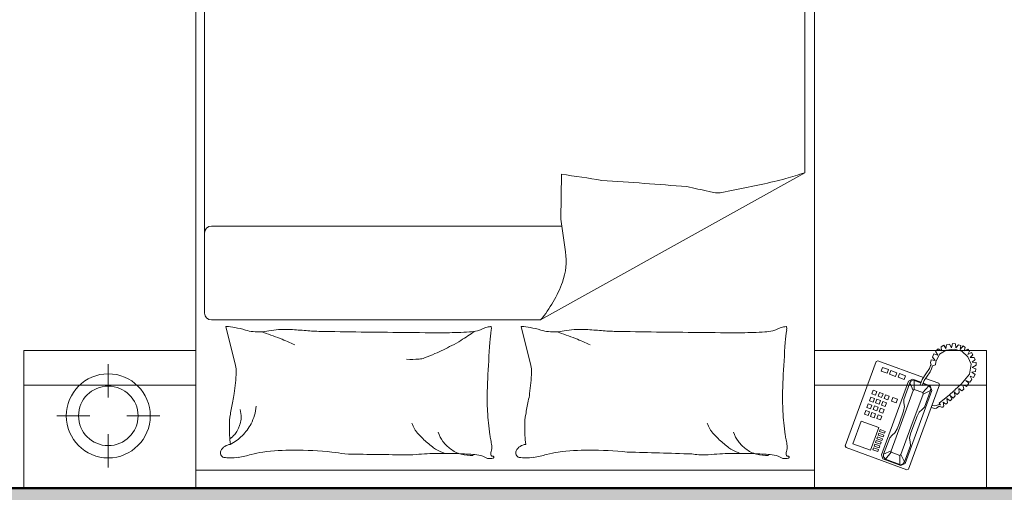
# Model space of a CAD drawing. Units: inches. Extents: x -7 to 1228, y -146 to 1091.
# Tile 45 of 88: x 81 to 169, y 574 to 616. Entities that reach past the tile are written whole.
import ezdxf

# ---------------------------------------------------------------- set-up
doc = ezdxf.new("R2010")
doc.units = ezdxf.units.IN
for name, color, linetype, lineweight in [('A-FURN', 8, 'Continuous', 18), ('A-WALL', 7, 'Continuous', 50), ('A-WALL-PATT', 251, 'Continuous', 13)]:
    doc.layers.add(name, color=color, linetype=linetype, lineweight=lineweight)
doc.styles.add('DIM_FONT', font='SIMPLEX.shx', dxfattribs={"width": 0.8})

# ---------------------------------------------------------------- blocks, each defined once
blk = doc.blocks.new('A$C4F634EDD')
for p, q in [((0, 2.6295), (0, 2.2295)), ((0.5, 2.6295), (0, 2.6295)), ((0.5, 2.6295), (2.3, 2.6295)), ((0.5, 0.5295), (0.5, 2.6295)), ((0.5, 2.2295), (0.5, 2.6295)), ((2.3, 2.6295), (2.3, 0.5295)), ((2.3, 2.6295), (2.8, 2.6295)), ((2.3, 2.2295), (2.3, 2.6295)), ((2.8, 2.6295), (2.8, 2.2295)), ((0.2457, 2.5697), (0.2457, 2.4733)), ((0.5, 2.5771), (2.3, 2.5771)), ((2.392, 2.5115), (2.5692, 2.5765)), ((2.4985, 2.5445), (2.5516, 2.564)), ((2.5062, 2.5454), (2.5487, 2.561)), ((2.5483, 2.5347), (2.5487, 2.561)), ((2.5487, 2.561), (2.5571, 2.56)), ((2.5615, 2.5536), (2.5514, 2.5318)), ((2.5516, 2.564), (2.5637, 2.5584)), ((2.5571, 2.56), (2.5615, 2.5536)), ((2.5615, 2.5536), (2.5791, 2.5058)), ((2.5637, 2.5584), (2.6418, 2.3458)), ((2.5692, 2.5765), (2.574, 2.5743)), ((2.574, 2.5743), (2.6638, 2.3298)), ((2.4842, 2.5232), (2.47, 2.518)), ((2.4862, 2.5179), (2.4842, 2.5232)), ((2.4946, 2.5331), (2.4985, 2.5445)), ((2.5734, 2.3187), (2.4946, 2.5331)), ((2.5062, 2.5454), (2.5004, 2.5392)), ((2.5004, 2.5392), (2.5013, 2.5315)), ((2.5013, 2.5315), (2.5188, 2.4836)), ((2.5013, 2.5315), (2.5231, 2.5214)), ((2.5235, 2.5256), (2.5062, 2.5454)), ((2.5231, 2.5214), (2.5235, 2.5256)), ((2.5523, 2.4417), (2.5231, 2.5214)), ((2.5483, 2.5347), (2.5235, 2.5256)), ((2.5514, 2.5318), (2.5483, 2.5347)), ((2.5807, 2.4521), (2.5514, 2.5318)), ((2.3898, 2.5066), (2.392, 2.5115)), ((2.4795, 2.2621), (2.3898, 2.5066)), ((2.412, 2.5007), (2.4634, 2.5196)), ((2.4361, 2.4352), (2.412, 2.5007)), ((2.4634, 2.5196), (2.4875, 2.454)), ((2.47, 2.518), (2.472, 2.5127)), ((2.472, 2.5127), (2.4862, 2.5179)), ((2.4881, 2.5126), (2.4739, 2.5074)), ((2.4739, 2.5074), (2.4759, 2.502)), ((2.4759, 2.502), (2.4901, 2.5073)), ((2.492, 2.5019), (2.4778, 2.4967)), ((2.4778, 2.4967), (2.4798, 2.4914)), ((2.4798, 2.4914), (2.494, 2.4966)), ((2.4901, 2.5073), (2.4881, 2.5126)), ((2.494, 2.4966), (2.492, 2.5019)), ((2.5788, 2.4956), (2.5767, 2.4848)), ((2.5791, 2.5058), (2.5788, 2.4956)), ((2.4959, 2.4913), (2.4817, 2.4861)), ((2.4817, 2.4861), (2.4837, 2.4808)), ((2.4837, 2.4808), (2.4979, 2.486)), ((2.4998, 2.4807), (2.4856, 2.4755)), ((2.4856, 2.4755), (2.4876, 2.4702)), ((2.4876, 2.4702), (2.5018, 2.4754)), ((2.5037, 2.47), (2.4895, 2.4648)), ((2.4895, 2.4648), (2.4915, 2.4595)), ((2.4915, 2.4595), (2.5057, 2.4647)), ((2.4979, 2.486), (2.4959, 2.4913)), ((2.5018, 2.4754), (2.4998, 2.4807)), ((2.5057, 2.4647), (2.5037, 2.47)), ((2.5188, 2.4836), (2.5256, 2.4761)), ((2.5256, 2.4761), (2.5342, 2.4692)), ((2.5342, 2.4692), (2.5405, 2.4574)), ((2.5767, 2.4848), (2.5795, 2.4717)), ((2.5795, 2.4717), (2.586, 2.454)), ((2.4875, 2.454), (2.4361, 2.4352)), ((2.5405, 2.4574), (2.547, 2.4397)), ((2.5594, 2.4061), (2.547, 2.4397)), ((2.5523, 2.4417), (2.5875, 2.346)), ((2.5807, 2.4521), (2.6158, 2.3564)), ((2.5984, 2.4204), (2.586, 2.454)), ((0.0957, 2.4197), (0.192, 2.4197)), ((0.2994, 2.4197), (0.3957, 2.4197)), ((2.4457, 2.4146), (2.4563, 2.4185)), ((2.4496, 2.4039), (2.4457, 2.4146)), ((2.4602, 2.4078), (2.4496, 2.4039)), ((2.4563, 2.4185), (2.4602, 2.4078)), ((2.4634, 2.4211), (2.474, 2.425)), ((2.4673, 2.4104), (2.4634, 2.4211)), ((2.4779, 2.4143), (2.4673, 2.4104)), ((2.474, 2.425), (2.4779, 2.4143)), ((2.4811, 2.4276), (2.4917, 2.4315)), ((2.485, 2.4169), (2.4811, 2.4276)), ((2.4956, 2.4208), (2.485, 2.4169)), ((2.4883, 2.4081), (2.4989, 2.412)), ((2.4922, 2.3975), (2.4883, 2.4081)), ((2.4917, 2.4315), (2.4956, 2.4208)), ((2.4989, 2.412), (2.5028, 2.4014)), ((2.5622, 2.393), (2.5594, 2.4061)), ((2.6047, 2.4086), (2.5984, 2.4204)), ((2.6133, 2.4017), (2.6047, 2.4086)), ((2.4528, 2.3951), (2.4635, 2.399)), ((2.4567, 2.3844), (2.4528, 2.3951)), ((2.4674, 2.3883), (2.4567, 2.3844)), ((2.46, 2.3756), (2.4706, 2.3795)), ((2.4635, 2.399), (2.4674, 2.3883)), ((2.4706, 2.4016), (2.4812, 2.4055)), ((2.4745, 2.3909), (2.4706, 2.4016)), ((2.4706, 2.3795), (2.4745, 2.3689)), ((2.4851, 2.3949), (2.4745, 2.3909)), ((2.4777, 2.3821), (2.4883, 2.386)), ((2.4816, 2.3715), (2.4777, 2.3821)), ((2.4812, 2.4055), (2.4851, 2.3949)), ((2.4883, 2.386), (2.4922, 2.3754)), ((2.5028, 2.4014), (2.4922, 2.3975)), ((2.4954, 2.3886), (2.5061, 2.3925)), ((2.4993, 2.378), (2.4954, 2.3886)), ((2.51, 2.3819), (2.4993, 2.378)), ((2.5061, 2.3925), (2.51, 2.3819)), ((2.5238, 2.3769), (2.538, 2.3821)), ((2.538, 2.3821), (2.5419, 2.3715)), ((2.5598, 2.372), (2.5601, 2.3822)), ((2.5601, 2.3822), (2.5622, 2.393)), ((2.6201, 2.3941), (2.6133, 2.4017)), ((2.6376, 2.3463), (2.6201, 2.3941)), ((2.6499, 2.3979), (2.6397, 2.3953)), ((2.6417, 2.39), (2.6488, 2.391)), ((2.6488, 2.391), (2.6538, 2.3895)), ((2.6551, 2.397), (2.6499, 2.3979)), ((2.6538, 2.3895), (2.6596, 2.388)), ((2.6627, 2.392), (2.6551, 2.397)), ((2.6596, 2.388), (2.6626, 2.3867)), ((2.6626, 2.3867), (2.6662, 2.388)), ((2.6692, 2.394), (2.6627, 2.392)), ((2.6662, 2.388), (2.6632, 2.3828)), ((2.6632, 2.3828), (2.6736, 2.3744)), ((2.6736, 2.3944), (2.6692, 2.394)), ((2.6765, 2.391), (2.6736, 2.3944)), ((2.6742, 2.3795), (2.6765, 2.391)), ((2.6824, 2.3858), (2.6742, 2.3795)), ((2.6873, 2.3815), (2.6824, 2.3858)), ((2.6853, 2.369), (2.6873, 2.3815)), ((0.2457, 2.366), (0.2457, 2.2697)), ((2.4639, 2.365), (2.46, 2.3756)), ((2.4745, 2.3689), (2.4639, 2.365)), ((2.4672, 2.3561), (2.4778, 2.36)), ((2.4711, 2.3455), (2.4672, 2.3561)), ((2.4817, 2.3494), (2.4711, 2.3455)), ((2.4778, 2.36), (2.4817, 2.3494)), ((2.4922, 2.3754), (2.4816, 2.3715)), ((2.4849, 2.3626), (2.4955, 2.3665)), ((2.4888, 2.352), (2.4849, 2.3626)), ((2.4994, 2.3559), (2.4888, 2.352)), ((2.4955, 2.3665), (2.4994, 2.3559)), ((2.5026, 2.3691), (2.5132, 2.373)), ((2.5065, 2.3585), (2.5026, 2.3691)), ((2.5171, 2.3624), (2.5065, 2.3585)), ((2.5132, 2.373), (2.5171, 2.3624)), ((2.5277, 2.3663), (2.5238, 2.3769)), ((2.5419, 2.3715), (2.5277, 2.3663)), ((2.5774, 2.3242), (2.5598, 2.372)), ((2.6154, 2.3522), (2.5905, 2.3431)), ((2.6158, 2.3564), (2.6154, 2.3522)), ((2.6154, 2.3522), (2.6327, 2.3324)), ((2.6376, 2.3463), (2.6158, 2.3564)), ((2.6736, 2.3744), (2.6922, 2.3593)), ((2.6946, 2.376), (2.6853, 2.369)), ((2.6922, 2.3593), (2.7051, 2.3473)), ((2.6995, 2.3713), (2.6946, 2.376)), ((2.695, 2.3603), (2.6995, 2.3713)), ((2.7031, 2.3682), (2.695, 2.3603)), ((2.7096, 2.3616), (2.7031, 2.3682)), ((2.7062, 2.351), (2.7096, 2.3616)), ((2.7147, 2.3578), (2.7062, 2.351)), ((2.7214, 2.3517), (2.7147, 2.3578)), ((2.7196, 2.34), (2.7214, 2.3517)), ((0, 2.3301), (0.5, 2.3301)), ((2.8, 2.3301), (2.3, 2.3301)), ((2.5774, 2.3242), (2.5875, 2.346)), ((2.5818, 2.3178), (2.5774, 2.3242)), ((2.6104, 2.3222), (2.5855, 2.3131)), ((2.5875, 2.346), (2.5905, 2.3431)), ((2.5905, 2.3431), (2.5901, 2.3168)), ((2.5901, 2.3168), (2.6097, 2.324)), ((2.613, 2.3312), (2.6077, 2.3293)), ((2.6077, 2.3293), (2.6135, 2.3141)), ((2.6192, 2.3174), (2.613, 2.3312)), ((2.6153, 2.3261), (2.6327, 2.3324)), ((2.6369, 2.332), (2.6161, 2.3243)), ((2.6616, 2.3249), (2.6234, 2.3109)), ((2.6327, 2.3324), (2.6385, 2.3386)), ((2.6418, 2.3458), (2.6369, 2.332)), ((2.6385, 2.3386), (2.6376, 2.3463)), ((2.6638, 2.3298), (2.6616, 2.3249)), ((2.7051, 2.3473), (2.7079, 2.3475)), ((2.7079, 2.3475), (2.7079, 2.3443)), ((2.7079, 2.3443), (2.727, 2.3277)), ((2.7286, 2.3466), (2.7196, 2.34)), ((2.727, 2.3277), (2.7512, 2.2983)), ((2.7346, 2.3423), (2.7286, 2.3466)), ((2.732, 2.3295), (2.7346, 2.3423)), ((2.7423, 2.3345), (2.732, 2.3295)), ((2.7406, 2.3172), (2.7495, 2.325)), ((2.7519, 2.3218), (2.7406, 2.3172)), ((2.7495, 2.325), (2.7423, 2.3345)), ((2.7575, 2.3144), (2.7519, 2.3218)), ((2.6172, 2.3086), (2.4844, 2.2599)), ((2.5114, 2.2959), (2.4936, 2.2894)), ((2.5153, 2.2853), (2.5114, 2.2959)), ((2.5362, 2.305), (2.5185, 2.2985)), ((2.5185, 2.2985), (2.5224, 2.2879)), ((2.5224, 2.2879), (2.5401, 2.2944)), ((2.5401, 2.2944), (2.5362, 2.305)), ((2.561, 2.3141), (2.5433, 2.3076)), ((2.5433, 2.3076), (2.5472, 2.297)), ((2.5472, 2.297), (2.5649, 2.3035)), ((2.5649, 2.3035), (2.561, 2.3141)), ((2.5855, 2.3131), (2.5734, 2.3187)), ((2.5901, 2.3168), (2.5818, 2.3178)), ((2.6135, 2.3141), (2.6244, 2.2977)), ((2.626, 2.3069), (2.6192, 2.3174)), ((2.6244, 2.2977), (2.6349, 2.2825)), ((2.6365, 2.2916), (2.626, 2.3069)), ((2.6407, 2.2834), (2.6365, 2.2916)), ((2.7512, 2.2983), (2.756, 2.2695)), ((2.7526, 2.3045), (2.7575, 2.3144)), ((2.7622, 2.308), (2.7526, 2.3045)), ((2.7574, 2.2924), (2.7673, 2.2997)), ((2.7687, 2.2905), (2.7574, 2.2924)), ((2.7673, 2.2997), (2.7622, 2.308)), ((0.5953, 2.1912), (0.616, 2.2738)), ((1.4546, 2.1912), (1.4752, 2.2738)), ((2.4936, 2.2894), (2.4976, 2.2788)), ((2.4976, 2.2788), (2.5153, 2.2853)), ((2.6349, 2.2825), (2.638, 2.273)), ((2.6399, 2.2712), (2.6374, 2.2659)), ((2.6374, 2.2659), (2.6398, 2.257)), ((2.638, 2.273), (2.6399, 2.2712)), ((2.6438, 2.2739), (2.6407, 2.2834)), ((2.6519, 2.2716), (2.6438, 2.2739)), ((2.6535, 2.2628), (2.6519, 2.2716)), ((2.6636, 2.2409), (2.6535, 2.2628)), ((2.756, 2.2695), (2.7459, 2.2483)), ((2.7587, 2.279), (2.7699, 2.2828)), ((2.7708, 2.2725), (2.7587, 2.279)), ((2.759, 2.2637), (2.7706, 2.2643)), ((2.7676, 2.2559), (2.759, 2.2637)), ((2.7699, 2.2828), (2.7687, 2.2905)), ((2.7706, 2.2643), (2.7708, 2.2725)), ((2.4844, 2.2599), (2.4795, 2.2621)), ((2.6398, 2.257), (2.6509, 2.259)), ((2.6509, 2.259), (2.6431, 2.2492)), ((2.6431, 2.2492), (2.6473, 2.2398)), ((2.6473, 2.2398), (2.6592, 2.2429)), ((2.6592, 2.2429), (2.6521, 2.2314)), ((2.6836, 2.2287), (2.6636, 2.2409)), ((2.7459, 2.2483), (2.7284, 2.2317)), ((2.7509, 2.2314), (2.7459, 2.2418)), ((2.7459, 2.2418), (2.7568, 2.2352)), ((2.7529, 2.2505), (2.7645, 2.2498)), ((2.7607, 2.2424), (2.7529, 2.2505)), ((2.7568, 2.2352), (2.7607, 2.2424)), ((2.7645, 2.2498), (2.7676, 2.2559)), ((0, 2.2295), (0.5, 2.2295)), ((2.8, 2.2295), (2.3, 2.2295)), ((2.6521, 2.2314), (2.6598, 2.2248)), ((2.6598, 2.2248), (2.6697, 2.2309)), ((2.6697, 2.2309), (2.6684, 2.219)), ((2.6684, 2.219), (2.6761, 2.2145)), ((2.6761, 2.2145), (2.6821, 2.2237)), ((2.6821, 2.2237), (2.6843, 2.2135)), ((2.7063, 2.2256), (2.6836, 2.2287)), ((2.6843, 2.2135), (2.6927, 2.2117)), ((2.6927, 2.2117), (2.6986, 2.222)), ((2.6986, 2.222), (2.7019, 2.2098)), ((2.7019, 2.2098), (2.7102, 2.2104)), ((2.7284, 2.2317), (2.7063, 2.2256)), ((2.7102, 2.2104), (2.7113, 2.2218)), ((2.7113, 2.2218), (2.7192, 2.2137)), ((2.7192, 2.2137), (2.7255, 2.2152)), ((2.7255, 2.2152), (2.7242, 2.2265)), ((2.7242, 2.2265), (2.7324, 2.2165)), ((2.7324, 2.2165), (2.7386, 2.2208)), ((2.7386, 2.2208), (2.7354, 2.2306)), ((2.7354, 2.2306), (2.7462, 2.2264)), ((2.7462, 2.2264), (2.7509, 2.2314)), ((0.5878, 2.1612), (0.5953, 2.1912)), ((1.4471, 2.1612), (1.4546, 2.1912)), ((0.5258, 2.121), (0.5258, 0.5617)), ((1.5035, 2.141), (0.5458, 2.141)), ((1.5035, 2.141), (2.2716, 1.7136)), ((1.576, 1.9433), (1.5624, 1.8479)), ((0.5458, 1.8684), (1.5653, 1.8684)), ((1.5624, 1.8479), (1.5641, 1.7178)), ((2.2716, 0.5617), (2.2716, 1.7136))]:
    blk.add_line(p, q)
for radius in [0.1222, 0.0865]:
    blk.add_circle((0.2457, 2.4197), radius)
for centre, radius, start, end in [((0.5848, 2.5274), 0.0131, 101.2724, 206.5805), ((0.6036, 2.5368), 0.0342, 206.5805, 265.5998), ((0.5999, 2.4516), 0.0904, 90, 101.2724), ((0.5999, 2.3808), 0.1611, 81.5628, 90), ((0.5788, 2.2388), 0.3048, 74.256, 81.5628), ((0.7272, 2.7653), 0.2422, 254.256, 262.4531), ((0.7851, 3.2019), 0.6827, 262.4531, 270), ((0.7851, 3.5682), 1.049, 270, 276.0867), ((0.8402, 3.0514), 0.5293, 276.0867, 280.1899), ((1.1602, -8.1346), 10.6675, 90.30153, 91.21582), ((1.1169, 2.2433), 0.2897, 85.1982, 92.5386), ((1.2142, 3.4021), 0.8732, 265.1982, 269.4243), ((1.3082, 2.3102), 0.234, 110.8603, 117.2396), ((1.2204, 4.0232), 1.4943, 269.4243, 271.9079), ((1.2995, 2.4357), 0.0992, 105.9352, 126.0864), ((1.2429, 3.3501), 0.8208, 271.9079, 275.2592), ((1.2995, 2.4357), 0.0992, 85.7841, 105.9352), ((1.3132, 2.5864), 0.0539, 275.2592, 300.6513), ((1.3554, 2.5152), 0.0289, 85.6975, 120.6513), ((1.3556, 2.519), 0.0251, 68.2117, 85.6975), ((1.3739, 2.5288), 0.0156, 158.0096, 201.421), ((1.3634, 2.533), 0.00428, 78.1069, 158.0096), ((1.3288, 2.5111), 0.0328, 351.8665, 21.421), ((1.3647, 2.5395), 0.00232, 258.1069, 19.564), ((1.3637, 2.5391), 0.00342, 19.564, 68.2117), ((1.444, 2.5274), 0.0131, 101.2724, 206.5805), ((1.4628, 2.5368), 0.0342, 206.5805, 265.5998), ((1.4591, 2.4516), 0.0904, 90, 101.2724), ((1.4591, 2.3808), 0.1611, 81.5628, 90), ((1.438, 2.2388), 0.3048, 74.256, 81.5628), ((1.5865, 2.7653), 0.2422, 254.256, 262.4531), ((1.6443, 3.2019), 0.6827, 262.4531, 270), ((1.6443, 3.5682), 1.049, 270, 276.0867), ((1.4785, 15.4878), 12.9656, 271.22425, 272.05324), ((1.97, 2.3805), 0.1524, 92.5386, 100.1899), ((1.9761, 2.2433), 0.2897, 85.1982, 92.5386), ((2.0734, 3.4021), 0.8732, 265.1982, 269.4243), ((2.1674, 2.3102), 0.234, 110.8603, 117.2396), ((2.0797, 4.0232), 1.4943, 269.4243, 271.9079), ((2.1588, 2.4357), 0.0992, 105.9352, 126.0864), ((2.1021, 3.3501), 0.8208, 271.9079, 275.2592), ((2.1588, 2.4357), 0.0992, 85.7841, 105.9352), ((2.1724, 2.5864), 0.0539, 275.2592, 300.6513), ((2.2146, 2.5152), 0.0289, 85.6975, 120.6513), ((2.2149, 2.519), 0.0251, 68.2117, 85.6975), ((2.2331, 2.5288), 0.0156, 158.0096, 201.421), ((2.2226, 2.533), 0.00428, 78.1069, 158.0096), ((2.1881, 2.5111), 0.0328, 351.8665, 21.421), ((2.224, 2.5395), 0.00232, 258.1069, 19.564), ((2.2229, 2.5391), 0.00342, 19.564, 68.2117), ((1.0898, 2.4496), 0.4918, 173.7676, 180), ((0.5368, 2.3783), 0.1399, 45.0976, 62.7964), ((1.4317, 2.2032), 0.3916, 128.3886, 133.8115), ((1.2362, 2.45), 0.0768, 117.2396, 128.3886), ((1.2995, 2.4357), 0.0992, 143.8234, 161.5603), ((1.2995, 2.4357), 0.0992, 126.0864, 143.8234), ((1.1177, 2.5413), 0.246, 347.8905, 351.8665), ((1.949, 2.4496), 0.4918, 173.7676, 180), ((2.291, 2.2032), 0.3916, 128.3886, 133.8115), ((2.0954, 2.45), 0.0768, 117.2396, 128.3886), ((2.1588, 2.4357), 0.0992, 143.8234, 161.5603), ((2.1588, 2.4357), 0.0992, 126.0864, 143.8234), ((1.977, 2.5413), 0.246, 347.8905, 351.8665), ((0.5462, 2.4142), 0.0899, 41.4429, 53.7359), ((0.5741, 2.4389), 0.0526, 25.3551, 41.4429), ((0.5368, 2.3783), 0.1399, 27.3988, 45.0976), ((1.1799, 2.4341), 0.0493, 140.9651, 151.6832), ((1.3165, 2.3233), 0.2252, 133.8115, 140.9651), ((2.2605, 2.3525), 0.9131, 172.3191, 176.6313), ((1.5522, 2.448), 0.1983, 167.8905, 172.3191), ((2.0391, 2.4341), 0.0493, 140.9651, 151.6832), ((2.1757, 2.3233), 0.2252, 133.8115, 140.9651), ((3.1198, 2.3525), 0.9131, 172.3191, 176.6313), ((2.4114, 2.448), 0.1983, 167.8905, 172.3191), ((0.8019, 2.4496), 0.204, 180, 189.6844), ((0.4851, 2.3967), 0.1511, 21.8149, 25.3551), ((0.4345, 2.3765), 0.2056, 18.7799, 21.8149), ((0.576, 2.4246), 0.0562, 0, 18.7799), ((0.5368, 2.3783), 0.1399, 16.515, 27.3988), ((1.3127, 2.3625), 0.2002, 151.6832, 156.9972), ((1.6611, 2.4496), 0.204, 180, 189.6844), ((2.1719, 2.3625), 0.2002, 151.6832, 156.9972), ((1.4703, 2.5637), 0.882, 189.6844, 192.1984), ((0.5406, 2.4246), 0.0915, 345.3149, 0), ((0.5368, 2.3783), 0.1399, 5.6311, 16.515), ((2.0266, 2.3663), 0.6787, 176.6313, 181.6331), ((2.3295, 2.5637), 0.882, 189.6844, 192.1984), ((2.8858, 2.3663), 0.6787, 176.6313, 181.6331), ((0.2982, 2.3103), 0.3171, 8.0051, 12.1984), ((-0.0401, 2.2627), 0.6588, 2.6649, 8.0051), ((1.1575, 2.3103), 0.3171, 8.0051, 12.1984), ((0.8191, 2.2627), 0.6588, 2.6649, 8.0051), ((2.7128, 2.3859), 1.3652, 181.6331, 183.055), ((3.5721, 2.3859), 1.3652, 181.6331, 183.055), ((0.5503, 2.2902), 0.0677, 345.9548, 2.6649), ((14.9657, 3.0398), 13.6356, 183.05496, 183.50486), ((1.4096, 2.2902), 0.0677, 345.9548, 2.6649), ((15.8249, 3.0398), 13.6356, 183.05496, 183.50486), ((1.1303, 1.9835), 0.2721, 85.9172, 93.5552), ((1.1455, 2.197), 0.058, 69.3257, 85.9172), ((0.9871, 1.7772), 0.5066, 65.6735, 69.3257), ((0.6058, 0.9338), 1.4323, 63.5015, 65.6735), ((0.473, 2.8815), 0.7387, 293.4844, 295.3111), ((1.1054, 1.9358), 0.3126, 57.865, 63.5015), ((1.6762, 2.2258), 0.3212, 183.5049, 189.9984), ((1.3322, 2.8815), 0.7387, 293.4844, 295.3111), ((2.5355, 2.2258), 0.3212, 183.5049, 189.9984), ((0.473, 2.8815), 0.7387, 287.1982, 289.428), ((0.473, 2.8815), 0.7387, 289.428, 291.6577), ((0.473, 2.8815), 0.7387, 291.6577, 293.4844), ((1.2501, -19.8405), 22.0183, 90.37908, 91.01965), ((1.2012, -3.5404), 5.7185, 89.7135, 90.9704), ((1.224, 1.0141), 1.164, 86.426, 89.7135), ((0.8841, 1.5835), 0.7286, 54.1737, 57.865), ((1.3322, 2.8815), 0.7387, 287.1982, 289.428), ((1.3322, 2.8815), 0.7387, 289.428, 291.6577), ((1.3322, 2.8815), 0.7387, 291.6577, 293.4844), ((2.1093, -19.8405), 22.0183, 90.37908, 91.01965), ((2.0605, -3.5404), 5.7185, 89.7135, 90.9704), ((2.0833, 1.0141), 1.164, 86.426, 89.7135), ((0.5887, 2.1609), 0.000917, 165.9551, 274.0829), ((0.5695, 2.4301), 0.2708, 274.0829, 279.4841), ((0.5763, 2.3896), 0.2297, 279.4841, 287.3864), ((0.6807, 2.0561), 0.1197, 96.4341, 107.3864), ((0.6836, 2.0301), 0.1459, 78.4414, 96.4341), ((0.759, 2.3985), 0.2301, 258.4414, 272.7491), ((0.7026, 3.5718), 1.4048, 272.7491, 274.6176), ((0.9136, 0.9591), 1.2165, 92.6096, 94.6176), ((1.2875, 2.0302), 0.1459, 77.131, 86.426), ((1.3099, 2.1283), 0.0453, 62.7159, 77.131), ((1.3658, 2.2367), 0.0767, 242.7159, 253.7788), ((1.3688, 2.247), 0.0875, 253.7788, 262.8796), ((1.3581, 2.1615), 0.00132, 262.8796, 343.3022), ((1.3409, 2.1667), 0.0193, 343.3022, 9.9984), ((1.448, 2.1609), 0.000917, 165.9551, 274.0829), ((1.4288, 2.4301), 0.2708, 274.0829, 279.4841), ((1.4355, 2.3896), 0.2297, 279.4841, 287.3864), ((1.5399, 2.0561), 0.1197, 96.4341, 107.3864), ((1.5429, 2.0301), 0.1459, 78.4414, 96.4341), ((1.6182, 2.3985), 0.2301, 258.4414, 272.7491), ((1.5619, 3.5718), 1.4048, 272.7491, 274.6176), ((1.7729, 0.9591), 1.2165, 92.6096, 94.6176), ((2.1467, 2.0302), 0.1459, 77.131, 86.426), ((2.1691, 2.1283), 0.0453, 62.7159, 77.131), ((2.2251, 2.2367), 0.0767, 242.7159, 253.7788), ((2.2281, 2.247), 0.0875, 253.7788, 262.8796), ((2.2174, 2.1615), 0.00132, 262.8796, 343.3022), ((2.2001, 2.1667), 0.0193, 343.3022, 9.9984), ((0.5458, 2.121), 0.02, 90, 180), ((1.2147, 1.9017), 0.3751, 20.1488, 39.6445), ((1.3977, 1.9688), 0.1801, 351.8644, 20.1488), ((0.5458, 1.8884), 0.02, 180, 270), ((0.6102, 18.0525), 16.3521, 273.75703, 274.62393), ((1.4194, 4.2174), 2.5158, 281.6741, 283.1904), ((2.0378, 1.5789), 0.1942, 97.7304, 103.1904), ((2.0195, 1.7137), 0.0581, 79.2724, 97.7304), ((1.2737, -2.2227), 4.0646, 77.0745, 79.2724), ((1.0582, 5.4638), 3.7801, 277.692, 279.495), ((2.0359, 1.0981), 0.6574, 74.0648, 77.0745), ((1.7125, -0.0344), 1.8351, 72.2636, 74.0648)]:
    blk.add_arc(centre, radius, start, end)
at = {"style": 'DIM_FONT', "width": 0.8, "flags": 9}
for tag, p in [('YSIZE', (0.5, 2.6295)), ('XSIZE', (0.5, 2.6295)), ('XSIZE', (2.2985, 2.6295)), ('YSIZE', (2.2985, 2.6295))]:
    blk.add_attdef(tag, p, '', height=0.0005, dxfattribs=at)

msp = doc.modelspace()

# ---------------------------------------------------------------- hatches: boundary and pattern name
at = {"layer": 'A-WALL-PATT'}
h = msp.add_hatch(color=256, dxfattribs=at)
h.dxf.hatch_style = 1
h.paths.add_polyline_path([(69, 568), (60, 568), (60, 493), (63.289, 493), (69, 493)])
h.paths.add_polyline_path([(69, 662.405), (60, 662.405), (60, 586), (69, 586)], flags=17)
h.paths.add_polyline_path([(69, 723), (184, 723), (184, 734), (179, 734), (179, 728), (69, 728), (69, 741.623), (60, 741.623), (60, 698.405), (69, 698.405)], flags=17)
h.paths.add_polyline_path([(69, 782), (231, 782), (231, 728), (231, 723), (231, 586), (236, 586), (236, 787), (69, 787), (69, 800.126), (60, 800.126), (60, 765.623), (69, 765.623)])
h.paths.add_polyline_path([(184, 842), (189, 842), (189, 848), (173, 848), (173, 842), (179, 842), (179, 787), (184, 787)])
h.paths.add_polyline_path([(118.22, 69), (69, 69), (69, 60), (118.22, 60)])
h.paths.add_polyline_path([(227, 69), (154.22, 69), (154.22, 60), (227, 60)])
h.paths.add_polyline_path([(236, 60), (232.711, 60), (227, 60), (227, 36), (236, 36)])
h.paths.add_polyline_path([(389, 60), (380, 60), (380, 36), (389, 36)])
h.paths.add_polyline_path([(384, 181), (380, 181), (380, 115), (380, 78), (384, 78)])
h.paths.add_polyline_path([(380, 115), (334.547, 115), (334.547, 109), (380, 109)])
h.paths.add_polyline_path([(274.547, 115), (236, 115), (236, 201), (232.711, 201), (231, 201), (231, 78), (236, 78), (236, 109), (274.547, 109)])
h.paths.add_polyline_path([(69, 123), (60, 123), (60, 78), (69, 78)])
h.paths.add_polyline_path([(69, 201), (60, 201), (60, 159), (69, 159)])
h.paths.add_polyline_path([(143, 219), (69, 219), (69, 213), (143, 213)], flags=17)
h.paths.add_polyline_path([(189, 219), (184, 219), (184, 274), (231, 274), (231, 219), (236, 219), (236, 279), (184, 279), (184, 297), (179, 297), (179, 279), (69, 279), (69, 290.912), (60, 290.912), (60, 262.179), (69, 262.179), (69, 274), (179, 274), (179, 219), (173, 219), (173, 213), (189, 213)])
h.paths.add_polyline_path([(69, 238.179), (60, 238.179), (60, 219), (69, 219)], flags=17)
h.paths.add_polyline_path([(69, 333), (60, 333), (60, 314.912), (69, 314.912), (69, 316.965)])
h.paths.add_polyline_path([(190, 338), (184, 338), (69, 338), (69, 333), (179, 333), (179, 327), (184, 327), (184, 333.021), (190, 333.046)])
h.paths.add_polyline_path([(69, 386.806), (60, 386.806), (60, 351), (69, 351)])
h.paths.add_polyline_path([(69, 475), (60, 475), (60, 422.806), (69, 422.806)])
h.paths.add_polyline_path([(236, 475), (231, 475), (231, 351.238), (236, 351.238)])
h.paths.add_polyline_path([(384, 475), (380, 475), (380, 362), (384, 362)])
h.paths.add_polyline_path([(547, 307), (439, 307), (439, 356), (445, 356), (445, 362), (433, 362), (433, 307), (380, 307), (380, 244), (380, 241), (384, 241), (384, 301), (433, 301), (433, 277), (439, 277), (439, 301), (547, 301)])
h.paths.add_polyline_path([(547, 241), (439, 241), (439, 247), (433, 247), (433, 235), (547, 235)])
h.paths.add_polyline_path([(450, 69), (440.286, 69), (424.889, 69), (389, 69), (389, 60), (450, 60)])
h.paths.add_polyline_path([(547, 69), (486, 69), (486, 60), (547, 60)])
h.paths.add_polyline_path([(556, 148.268), (547, 148.268), (547, 78), (556, 78)])
h.paths.add_polyline_path([(556, 223), (547, 223), (547, 195), (547, 184.268), (556, 184.268)])
h.paths.add_polyline_path([(556, 311.192), (547, 311.192), (547, 273.075), (556, 273.075)])
h.paths.add_polyline_path([(556, 344), (552.711, 344), (547, 344), (547, 335.192), (556, 335.192)])
h.paths.add_polyline_path([(556, 249.075), (547, 249.075), (547, 241), (556, 241)])
h.paths.add_polyline_path([(547, 362), (475, 362), (475, 356), (547, 356)], flags=0)
h.paths.add_polyline_path([(556, 399.621), (547, 399.621), (547, 362), (556, 362)])
h.paths.add_polyline_path([(556, 475), (547, 475), (547, 435.621), (556, 435.621)])
h.paths.add_polyline_path([(547, 493), (389, 493), (389, 487), (547, 487)])
h.paths.add_polyline_path([(380, 493), (278, 493), (278, 487), (380, 487)])
h.paths.add_polyline_path([(227, 493), (69, 493), (69, 487), (227, 487)])
h.paths.add_polyline_path([(643, 122.445), (634, 122.445), (634, 78), (643, 78)])
h.paths.add_polyline_path([(702.5, 69), (692.786, 69), (677.389, 69), (643, 69), (643, 60), (702.5, 60)])
h.paths.add_polyline_path([(798, 69), (738.5, 69), (738.5, 60), (798, 60)])
h.paths.add_polyline_path([(807, 60), (803.711, 60), (798, 60), (798, 36), (807, 36)])
h.paths.add_polyline_path([(807, 109), (846.751, 109), (846.751, 115), (807, 115), (807, 159), (802, 159), (802, 78), (807, 78)])
h.paths.add_polyline_path([(807, 201), (802, 201), (802, 195), (807, 195)])
h.paths.add_polyline_path([(643, 201), (634, 201), (634, 158.445), (643, 158.445)])
h.paths.add_polyline_path([(756, 225), (751, 225), (751, 219), (643, 219), (643, 213), (756, 213)])
h.paths.add_polyline_path([(643, 240.848), (634, 240.848), (634, 219), (643, 219)])
h.paths.add_polyline_path([(643, 274), (643, 288.629), (634, 288.629), (634, 264.848), (643, 264.848)])
h.paths.add_polyline_path([(802, 279), (756, 279), (756, 297), (751, 297), (751, 279), (643, 279), (643, 274), (751, 274), (751, 255), (756, 255), (756, 274), (802, 274)])
h.paths.add_polyline_path([(807, 333), (803.711, 333), (802, 333), (802, 279), (802, 274), (802, 219), (807, 219)])
h.paths.add_polyline_path([(956, 182), (951, 182), (951, 115), (906.751, 115), (906.751, 109), (951, 109), (951, 78), (956, 78)])
h.paths.add_polyline_path([(960, 60), (951, 60), (951, 36), (960, 36)])
h.paths.add_polyline_path([(1021, 69), (1005.781, 69), (960, 69), (960, 60), (1021, 60)])
h.paths.add_polyline_path([(956, 224), (951, 224), (951, 218), (956, 218)])
h.paths.add_polyline_path([(956, 302), (1004, 302), (1004, 278), (1010, 278), (1010, 302), (1118, 302), (1118, 290.809), (1127, 290.809), (1127, 326.968), (1118, 326.968), (1118, 320.966), (1118, 307), (1010, 307), (1010, 356), (1016, 356), (1016, 362), (1004, 362), (1004, 307), (951, 307), (951, 244), (951, 242), (954.289, 242), (956, 242)])
h.paths.add_polyline_path([(643, 333), (634, 333), (634, 312.629), (643, 312.629), (643, 316.965)])
h.paths.add_polyline_path([(756, 338), (643, 338), (643, 333), (751, 333), (751, 327), (756, 327)])
h.paths.add_polyline_path([(643, 388), (634, 388), (634, 351), (643, 351)])
h.paths.add_polyline_path([(807, 357), (802, 357), (802, 351), (807, 351)])
h.paths.add_polyline_path([(807, 475), (802, 475), (802, 393), (807, 393)])
h.paths.add_polyline_path([(643, 475), (634, 475), (634, 424), (643, 424)])
h.paths.add_polyline_path([(798, 493), (643, 493), (643, 487), (798, 487)])
h.paths.add_polyline_path([(634, 493), (556, 493), (556, 487), (634, 487)])
h.paths.add_polyline_path([(813, 493), (807, 493), (807, 487), (813, 487)])
h.paths.add_polyline_path([(951, 493), (849, 493), (849, 487), (951, 487)])
h.paths.add_polyline_path([(956, 484), (951, 484), (951, 374), (956, 374)])
h.paths.add_polyline_path([(1109, 493), (969, 493), (969, 487), (1109, 487)])
h.paths.add_polyline_path([(1127, 484), (1118, 484), (1118, 450.641), (1127, 450.641)])
h.paths.add_polyline_path([(1127, 414.641), (1118, 414.641), (1118, 365), (1127, 365)])
h.paths.add_polyline_path([(1109, 362), (1046, 362), (1046, 356), (1109, 356)], flags=17)
h.paths.add_polyline_path([(1127, 356), (1123.454, 356), (1118, 356), (1118, 350.968), (1127, 350.968)], flags=0)
h.paths.add_polyline_path([(1127, 266.809), (1118, 266.809), (1118, 262.361), (1118, 242), (1127, 242)], flags=17)
h.paths.add_polyline_path([(1118, 242), (1010, 242), (1010, 248), (1004, 248), (1004, 237), (1118, 237)])
h.paths.add_polyline_path([(1127, 224), (1118, 224), (1118, 170), (1127, 170)])
h.paths.add_polyline_path([(1127, 134), (1118, 134), (1118, 78), (1127, 78)])
h.paths.add_polyline_path([(1118, 69), (1057, 69), (1057, 60), (1118, 60)])
h.paths.add_polyline_path([(227, 571.546), (227, 574), (69, 574), (69, 568), (227, 568)])
h.paths.add_polyline_path([(380, 571.546), (380, 574), (278, 574), (278, 568), (380, 568)])
h.paths.add_polyline_path([(242, 574), (236, 574), (236, 568), (242, 568)])
h.paths.add_polyline_path([(547, 571.546), (547, 574), (389, 574), (389, 568), (547, 568)])
h.paths.add_polyline_path([(384, 733), (380, 733), (380, 586), (384, 586)])
h.paths.add_polyline_path([(556, 646), (634, 646), (634, 655), (547, 655), (547, 586), (556, 586)])
h.paths.add_polyline_path([(634, 574), (556, 574), (556, 568), (634, 568)])
h.paths.add_polyline_path([(643, 655), (634, 655), (634, 586), (643, 586)])
h.paths.add_polyline_path([(798, 574), (643, 574), (643, 568), (798, 568)])
h.paths.add_polyline_path([(643, 663.854), (634, 663.854), (634, 655), (643, 655)])
h.paths.add_polyline_path([(556, 676.967), (547, 676.967), (547, 655), (556, 655)])
h.paths.add_polyline_path([(556, 733), (547, 733), (547, 712.967), (556, 712.967)])
h.paths.add_polyline_path([(643, 710), (634, 710), (634, 699.854), (643, 699.854)])
h.paths.add_polyline_path([(807, 668), (802, 668), (802, 586), (807, 586)])
h.paths.add_polyline_path([(951, 574), (849, 574), (849, 568), (951, 568)])
h.paths.add_polyline_path([(956, 691), (951, 691), (951, 577), (956, 577)])
h.paths.add_polyline_path([(1109, 574), (969, 574), (969, 568), (1109, 568)])
h.paths.add_polyline_path([(1127, 643.403), (1118, 643.403), (1118, 577), (1127, 577)])
h.paths.add_polyline_path([(1127, 568), (1123.454, 568), (1118, 568), (1118, 493), (1127, 493)])
h.paths.add_polyline_path([(1127, 733), (1118, 733), (1118, 679.403), (1127, 679.403)])
h.paths.add_polyline_path([(1127, 777.348), (1118, 777.348), (1118, 770.035), (1118, 751), (1127, 751)], flags=17)
h.paths.add_polyline_path([(1118, 751), (1010, 751), (1010, 757), (1004, 757), (1004, 745), (1118, 745)])
h.paths.add_polyline_path([(956, 811), (1004, 811), (1004, 787), (1010, 787), (1010, 811), (1017.874, 811), (1017.874, 811.627, -0.414214), (1018.247, 812), (1031.978, 812, -0.414214), (1032.351, 811.627), (1032.351, 811), (1118, 811), (1118, 801.348), (1127, 801.348), (1127, 834.685), (1118, 834.685), (1118, 830.238), (1118, 817), (1010, 817), (1010, 866), (1016, 866), (1016, 872), (1004, 872), (1004, 817), (956, 817), (956, 866), (951, 866), (951, 751), (954.289, 751), (956, 751)])
h.paths.add_polyline_path([(1118, 872), (1046, 872), (1046, 866), (1118, 866)], flags=17)
h.paths.add_polyline_path([(1127, 924.711), (1118, 924.711), (1118, 884), (1127, 884)])
h.paths.add_polyline_path([(1127, 866), (1123.711, 866), (1118, 866), (1118, 858.685), (1127, 858.685)], flags=17)
h.paths.add_polyline_path([(956, 983), (951, 983), (951, 952), (807, 952), (807, 983), (802, 983), (802, 902), (807, 902), (807, 946), (951, 946), (951, 884), (956, 884)])
h.paths.add_polyline_path([(807, 842), (802, 842), (802, 787), (756, 787), (756, 806), (751, 806), (751, 787), (643, 787), (643, 782), (751, 782), (751, 764), (756, 764), (756, 782), (802, 782), (802, 728), (807, 728)])
h.paths.add_polyline_path([(756, 848), (643, 848), (643, 842), (751, 842), (751, 836), (756, 836)])
h.paths.add_polyline_path([(756, 734), (751, 734), (751, 728), (643, 728), (643, 723), (756, 723)])
h.paths.add_polyline_path([(643, 749.791), (634, 749.791), (634, 728), (637.289, 728), (643, 728)])
h.paths.add_polyline_path([(643, 805.405), (634, 805.405), (634, 773.791), (643, 773.791)])
h.paths.add_polyline_path([(643, 896.663), (634, 896.663), (634, 860), (637.289, 860), (643, 860)])
h.paths.add_polyline_path([(643, 842), (634, 842), (634, 829.405), (643, 829.405)])
h.paths.add_polyline_path([(643, 983), (634, 983), (634, 932.663), (643, 932.663)])
h.paths.add_polyline_path([(1127, 983), (1118, 983), (1118, 960.711), (1127, 960.711)])
h.paths.add_polyline_path([(1118, 1001), (1077.525, 1001), (1077.525, 992), (1118, 992)])
h.paths.add_polyline_path([(1041.525, 1001), (960, 1001), (960, 992), (1041.525, 992)])
h.paths.add_polyline_path([(960, 1025), (951, 1025), (951, 1001), (954.289, 1001), (960, 1001)])
h.paths.add_polyline_path([(807, 1025), (798, 1025), (798, 1001), (807, 1001)])
h.paths.add_polyline_path([(798, 1001), (738.5, 1001), (738.5, 992), (798, 992)])
h.paths.add_polyline_path([(702.5, 1001), (643, 1001), (643, 992), (702.5, 992)])
h.paths.add_polyline_path([(547, 1001), (499.113, 1001), (499.113, 992), (547, 992)])
h.paths.add_polyline_path([(463.113, 1001), (389, 1001), (389, 992), (463.113, 992)])
h.paths.add_polyline_path([(389, 1025), (380, 1025), (380, 1022), (380, 1001), (383.289, 1001), (389, 1001)])
h.paths.add_polyline_path([(236, 1025), (227, 1025), (227, 1001), (236, 1001)])
h.paths.add_polyline_path([(236, 983), (231, 983), (231, 860), (236, 860)])
h.paths.add_polyline_path([(274.547, 952), (236, 952), (236, 946), (274.547, 946)])
h.paths.add_polyline_path([(380, 952), (334.547, 952), (334.547, 946), (380, 946)])
h.paths.add_polyline_path([(384, 983), (380, 983), (380, 884), (383.289, 884), (384, 884)])
h.paths.add_polyline_path([(227, 1001), (155.012, 1001), (155.012, 992), (162.875, 992), (227, 992)])
h.paths.add_polyline_path([(119.012, 1001), (69, 1001), (69, 992), (119.012, 992)])
h.paths.add_polyline_path([(69, 983), (60, 983), (60, 922.987), (69, 922.987)])
h.paths.add_polyline_path([(69, 886.987), (60, 886.987), (60, 860), (63.289, 860), (69, 860)])
h.paths.add_polyline_path([(143, 848), (69, 848), (69, 842), (143, 842)])

# ---------------------------------------------------------------- linework, layer by layer
at = {"layer": 'A-WALL'}
msp.add_line((231, 574), (69, 574), dxfattribs=at)

# ---------------------------------------------------------------- block references
at = {"layer": 'A-FURN', "xscale": -30.79356024027943, "yscale": 30.79356024027943, "zscale": 30.79356024027943, "rotation": 180}
msp.add_blockref('A$C4F634EDD', (81.405, 654.972), dxfattribs=at)

doc.saveas('drawing.dxf')
